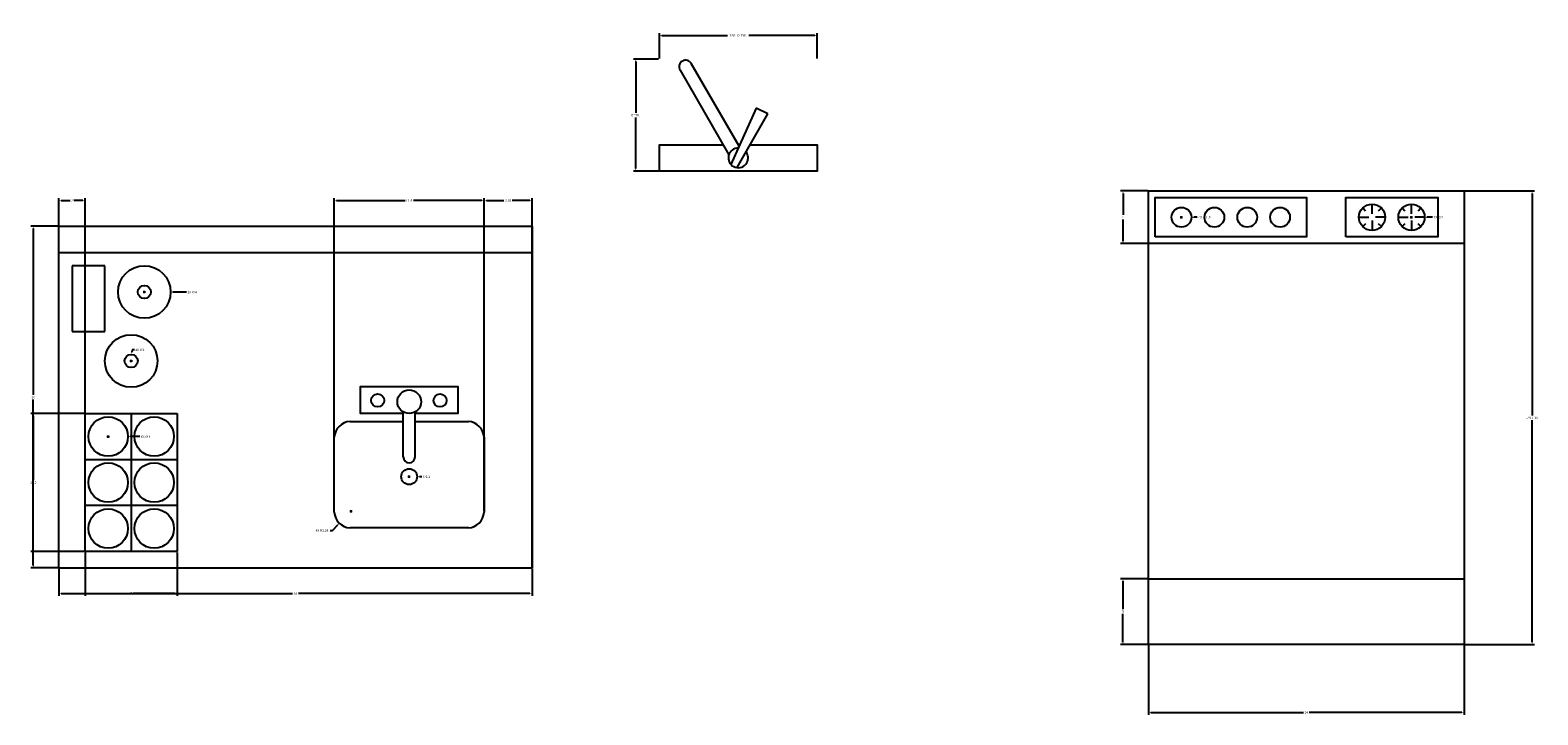
# Model space of a CAD drawing. Units: inches. Extents: x 821 to 2399, y 74 to 823.
# Tile 11 of 13: x 2026 to 2141, y 392 to 444. Entities that reach past the tile are written whole.
import ezdxf

# ---------------------------------------------------------------- set-up
doc = ezdxf.new("R2010")
doc.units = ezdxf.units.IN
doc.header["$MEASUREMENT"] = 0
doc.layers.get('0').update_dxf_attribs({"lineweight": 53})
for name, color, linetype, lineweight in [('A-ANNO-DIMS', 2, 'Continuous', 18), ('A-EQPM', 9, 'Continuous', 25), ('A-FLOR-CASE', 9, 'Continuous', 25), ('A-FLOR-FIXT', 8, 'Continuous', 25)]:
    doc.layers.add(name, color=color, linetype=linetype, lineweight=lineweight)
doc.styles.get("Standard").update_dxf_attribs({"font": 'arial.ttf'})
doc.dimstyles.get("Standard").update_dxf_attribs({"dimtxt": 0.18, "dimasz": 0.18, "dimexe": 0.18, "dimexo": 0.0625, "dimgap": 0.09, "dimtad": 0, "dimtih": 1, "dimtoh": 1, "dimdec": 4, "dimzin": 0, "dimdsep": 46, "dimtxsty": 'Standard', "dimcen": 0.09, "dimadec": 0, "dimazin": 0, "dimtfac": 1, "dimtdec": 4, "dimtofl": 0, "dimtmove": 0, "dimatfit": 3, "dimfxl": 1, "dimtolj": 1, "dimtzin": 0, "dimarcsym": 0})

# ---------------------------------------------------------------- blocks, each defined once
blk = doc.blocks.new('Faucet - single handle top')
for p, q in [((0.08, -0.26), (-2.26, -4.34)), ((-1.37, -4.79), (0.55, -0.5)), ((-0.06, -1.9), (3.57, -8.18)), ((4.43, -7.68), (0.72, -1.24)), ((-2.26, -4.34), (-1.37, -4.79))]:
    blk.add_line(p, q)
for points in [[(-0.92, -2), (-6, -2), (-6, 0), (6, 0), (6, -2), (1.16, -2)], [(-0.01, -2), (-0.12, -2)]]:
    blk.add_lwpolyline(points)
for centre, radius, start, end in [((0, -1), 0.75, 269.2246, 216.2304), ((4, -7.93), 0.5, 210, 30)]:
    blk.add_arc(centre, radius, start, end)
blk = doc.blocks.new('Dishwasher')
for p, q in [((17, 32.75), (17, 33.5)), ((20, 32.75), (20, 33.5)), ((16, 32.5), (16.75, 32.5)), ((16.3156, 33.1843), (16.5, 33)), ((17, 32.25), (17, 31.5)), ((18, 32.5), (17.25, 32.5)), ((17.5, 33), (17.6938, 33.1938)), ((19, 32.5), (19.75, 32.5)), ((19.3156, 33.1843), (19.5, 33)), ((20, 32.25), (20, 31.5)), ((21, 32.5), (20.25, 32.5)), ((20.5, 33), (20.6938, 33.1938)), ((16.5, 32), (16.2942, 31.7942)), ((17.7061, 31.7939), (17.5, 32)), ((19.5, 32), (19.2942, 31.7942)), ((20.7061, 31.7939), (20.5, 32)), ((24, 30.5), (0, 30.5)), ((0, 5), (24, 5))]:
    blk.add_line(p, q)
for points in [[(0, 0), (0, 34.5), (24, 34.5), (24, 0)], [(0.5, 31), (0.5, 34), (12, 34), (12, 31)], [(15, 31), (15, 34), (22, 34), (22, 31)]]:
    blk.add_lwpolyline(points, close=True)
for centre, radius in [((17, 32.5), 1), ((20, 32.5), 1), ((2.5, 32.5), 0.75), ((5, 32.5), 0.75), ((7.5, 32.5), 0.75), ((10, 32.5), 0.75)]:
    blk.add_circle(centre, radius)
blk = doc.blocks.new('*D36')
at = {"layer": 'A-ANNO-DIMS', "color": 0, "lineweight": -2, "transparency": 16777216}
for p, q in [((2074.05, 441.47), (2074.05, 443.39)), ((2074.23, 443.21), (2079.24, 443.21)), ((2085.87, 443.21), (2080.86, 443.21)), ((2086.05, 441.47), (2086.05, 443.39))]:
    blk.add_line(p, q, dxfattribs=at)
at = {"layer": 'A-ANNO-DIMS', "color": 0, "lineweight": 50, "transparency": 16777216}
for points in [[(2074.23, 443.24), (2074.23, 443.18), (2074.05, 443.21)], [(2085.87, 443.24), (2085.87, 443.18), (2086.05, 443.21)]]:
    blk.add_solid(points, dxfattribs=at)
at = {"layer": 'Defpoints', "color": 0, "lineweight": 50, "transparency": 16777216}
for p in [(2074.05, 443.21), (2074.05, 441.41), (2086.05, 441.41)]:
    blk.add_point(p, dxfattribs=at)
at = {"layer": 'A-ANNO-DIMS', "color": 0, "transparency": 16777216, "insert": (2080.05, 443.21), "char_height": 0.18, "attachment_point": 5}
blk.add_mtext('\\A1;TAP 12 TYP.', dxfattribs=at)
blk = doc.blocks.new('*D37')
at = {"layer": 'A-ANNO-DIMS', "color": 0, "lineweight": -2, "transparency": 16777216}
for p, q in [((2073.98, 441.41), (2072.07, 441.41)), ((2072.25, 441.23), (2072.25, 437.34)), ((2072.25, 433.09), (2072.25, 436.98)), ((2073.98, 432.91), (2072.07, 432.91))]:
    blk.add_line(p, q, dxfattribs=at)
at = {"layer": 'A-ANNO-DIMS', "color": 0, "lineweight": 50, "transparency": 16777216}
for points in [[(2072.22, 441.23), (2072.28, 441.23), (2072.25, 441.41)], [(2072.22, 433.09), (2072.28, 433.09), (2072.25, 432.91)]]:
    blk.add_solid(points, dxfattribs=at)
at = {"layer": 'Defpoints', "color": 0, "lineweight": 50, "transparency": 16777216}
for p in [(2074.05, 441.41), (2072.25, 432.91), (2074.05, 432.91)]:
    blk.add_point(p, dxfattribs=at)
at = {"layer": 'A-ANNO-DIMS', "color": 0, "transparency": 16777216, "insert": (2072.25, 437.16), "char_height": 0.18, "attachment_point": 5}
blk.add_mtext('\\A1;8 TYP.', dxfattribs=at)
blk = doc.blocks.new('*D76')
at = {"layer": 'A-ANNO-DIMS', "color": 0, "lineweight": -2, "transparency": 16777216}
for p, q in [((2135.34, 431.39), (2140.63, 431.39)), ((2140.45, 431.21), (2140.45, 414.32)), ((2140.45, 397.07), (2140.45, 413.96)), ((2135.34, 396.89), (2140.63, 396.89))]:
    blk.add_line(p, q, dxfattribs=at)
at = {"layer": 'A-ANNO-DIMS', "color": 0, "lineweight": 50, "transparency": 16777216}
for points in [[(2140.42, 431.21), (2140.48, 431.21), (2140.45, 431.39)], [(2140.42, 397.07), (2140.48, 397.07), (2140.45, 396.89)]]:
    blk.add_solid(points, dxfattribs=at)
at = {"layer": 'Defpoints', "color": 0, "lineweight": 50, "transparency": 16777216}
for p in [(2135.27, 431.39), (2140.45, 431.39), (2135.27, 396.89)]:
    blk.add_point(p, dxfattribs=at)
at = {"layer": 'A-ANNO-DIMS', "color": 0, "transparency": 16777216, "insert": (2140.45, 414.14), "char_height": 0.18, "attachment_point": 5}
blk.add_mtext('\\A1;UNIT 35', dxfattribs=at)
blk = doc.blocks.new('*D77')
at = {"layer": 'A-ANNO-DIMS', "color": 0, "lineweight": -2, "transparency": 16777216}
for p, q in [((2111.27, 396.83), (2111.27, 391.54)), ((2135.27, 396.83), (2135.27, 391.54)), ((2111.45, 391.72), (2123.05, 391.72)), ((2135.09, 391.72), (2123.49, 391.72))]:
    blk.add_line(p, q, dxfattribs=at)
at = {"layer": 'A-ANNO-DIMS', "color": 0, "lineweight": 50, "transparency": 16777216}
for points in [[(2111.45, 391.75), (2111.45, 391.69), (2111.27, 391.72)], [(2135.09, 391.75), (2135.09, 391.69), (2135.27, 391.72)]]:
    blk.add_solid(points, dxfattribs=at)
at = {"layer": 'Defpoints', "color": 0, "lineweight": 50, "transparency": 16777216}
for p in [(2111.27, 396.89), (2135.27, 396.89), (2135.27, 391.72)]:
    blk.add_point(p, dxfattribs=at)
at = {"layer": 'A-ANNO-DIMS', "color": 0, "transparency": 16777216, "insert": (2123.27, 391.72), "char_height": 0.18, "attachment_point": 5}
blk.add_mtext('\\A1;24', dxfattribs=at)
blk = doc.blocks.new('*D109')
at = {"layer": 'A-ANNO-DIMS', "color": 0, "lineweight": -2, "transparency": 16777216}
for p, q in [((2028.36, 402.64), (2028.36, 400.58)), ((2064.36, 402.64), (2064.36, 400.58)), ((2028.54, 400.76), (2046.14, 400.76)), ((2064.18, 400.76), (2046.58, 400.76))]:
    blk.add_line(p, q, dxfattribs=at)
at = {"layer": 'A-ANNO-DIMS', "color": 0, "lineweight": 50, "transparency": 16777216}
for points in [[(2028.54, 400.79), (2028.54, 400.73), (2028.36, 400.76)], [(2064.18, 400.79), (2064.18, 400.73), (2064.36, 400.76)]]:
    blk.add_solid(points, dxfattribs=at)
at = {"layer": 'Defpoints', "color": 0, "lineweight": 50, "transparency": 16777216}
for p in [(2028.36, 402.71), (2064.36, 402.71), (2064.36, 400.76)]:
    blk.add_point(p, dxfattribs=at)
at = {"layer": 'A-ANNO-DIMS', "color": 0, "transparency": 16777216, "insert": (2046.36, 400.76), "char_height": 0.18, "attachment_point": 5}
blk.add_mtext('\\A1;36', dxfattribs=at)
blk = doc.blocks.new('*D110')
at = {"layer": 'A-ANNO-DIMS', "color": 0, "lineweight": -2, "transparency": 16777216}
for p, q in [((2028.3, 428.71), (2026.23, 428.71)), ((2026.41, 428.53), (2026.41, 415.89)), ((2026.41, 402.89), (2026.41, 415.52)), ((2028.3, 402.71), (2026.23, 402.71))]:
    blk.add_line(p, q, dxfattribs=at)
at = {"layer": 'A-ANNO-DIMS', "color": 0, "lineweight": 50, "transparency": 16777216}
for points in [[(2026.38, 428.53), (2026.44, 428.53), (2026.41, 428.71)], [(2026.38, 402.89), (2026.44, 402.89), (2026.41, 402.71)]]:
    blk.add_solid(points, dxfattribs=at)
at = {"layer": 'Defpoints', "color": 0, "lineweight": 50, "transparency": 16777216}
for p in [(2026.41, 428.71), (2028.36, 428.71), (2028.36, 402.71)]:
    blk.add_point(p, dxfattribs=at)
at = {"layer": 'A-ANNO-DIMS', "color": 0, "transparency": 16777216, "insert": (2026.41, 415.71), "char_height": 0.18, "attachment_point": 5}
blk.add_mtext('\\A1;26', dxfattribs=at)
blk = doc.blocks.new('*D111')
at = {"layer": 'A-ANNO-DIMS', "color": 0, "lineweight": -2, "transparency": 16777216}
for p, q in [((2028.36, 402.77), (2028.36, 430.84)), ((2028.54, 430.66), (2029.21, 430.66)), ((2030.18, 430.66), (2029.51, 430.66)), ((2030.36, 404.02), (2030.36, 430.84))]:
    blk.add_line(p, q, dxfattribs=at)
at = {"layer": 'A-ANNO-DIMS', "color": 0, "lineweight": 50, "transparency": 16777216}
for points in [[(2028.54, 430.69), (2028.54, 430.63), (2028.36, 430.66)], [(2030.18, 430.69), (2030.18, 430.63), (2030.36, 430.66)]]:
    blk.add_solid(points, dxfattribs=at)
at = {"layer": 'Defpoints', "color": 0, "lineweight": 50, "transparency": 16777216}
for p in [(2030.36, 430.66), (2030.36, 403.96), (2028.36, 402.71)]:
    blk.add_point(p, dxfattribs=at)
at = {"layer": 'A-ANNO-DIMS', "color": 0, "transparency": 16777216, "insert": (2029.36, 430.66), "char_height": 0.18, "attachment_point": 5}
blk.add_mtext('\\A1;2', dxfattribs=at)
blk = doc.blocks.new('*D112')
at = {"layer": 'A-ANNO-DIMS', "color": 0, "lineweight": -2, "transparency": 16777216}
for p, q in [((2030.36, 403.89), (2030.36, 400.58)), ((2037.36, 403.89), (2037.36, 400.58)), ((2030.54, 400.76), (2033.72, 400.76)), ((2037.18, 400.76), (2034.01, 400.76))]:
    blk.add_line(p, q, dxfattribs=at)
at = {"layer": 'A-ANNO-DIMS', "color": 0, "lineweight": 50, "transparency": 16777216}
for points in [[(2030.54, 400.79), (2030.54, 400.73), (2030.36, 400.76)], [(2037.18, 400.79), (2037.18, 400.73), (2037.36, 400.76)]]:
    blk.add_solid(points, dxfattribs=at)
at = {"layer": 'Defpoints', "color": 0, "lineweight": 50, "transparency": 16777216}
for p in [(2030.36, 403.96), (2037.36, 403.96), (2037.36, 400.76)]:
    blk.add_point(p, dxfattribs=at)
at = {"layer": 'A-ANNO-DIMS', "color": 0, "transparency": 16777216, "insert": (2033.86, 400.76), "char_height": 0.18, "attachment_point": 5}
blk.add_mtext('\\A1;7', dxfattribs=at)
blk = doc.blocks.new('*D113')
at = {"layer": 'A-ANNO-DIMS', "color": 0, "lineweight": -2, "transparency": 16777216}
for p, q in [((2030.3, 414.46), (2026.23, 414.46)), ((2026.41, 414.28), (2026.41, 409.39)), ((2026.41, 404.14), (2026.41, 409.02)), ((2030.3, 403.96), (2026.23, 403.96))]:
    blk.add_line(p, q, dxfattribs=at)
at = {"layer": 'A-ANNO-DIMS', "color": 0, "lineweight": 50, "transparency": 16777216}
for points in [[(2026.38, 414.28), (2026.44, 414.28), (2026.41, 414.46)], [(2026.38, 404.14), (2026.44, 404.14), (2026.41, 403.96)]]:
    blk.add_solid(points, dxfattribs=at)
at = {"layer": 'Defpoints', "color": 0, "lineweight": 50, "transparency": 16777216}
for p in [(2026.41, 414.46), (2030.36, 414.46), (2030.36, 403.96)]:
    blk.add_point(p, dxfattribs=at)
at = {"layer": 'A-ANNO-DIMS', "color": 0, "transparency": 16777216, "insert": (2026.41, 409.21), "char_height": 0.18, "attachment_point": 5}
blk.add_mtext('\\A1;10.5', dxfattribs=at)
blk = doc.blocks.new('*D114')
at = {"layer": 'A-ANNO-DIMS', "color": 0, "lineweight": -2, "transparency": 16777216}
for p, q in [((2049.31, 407.02), (2049.31, 430.84)), ((2049.49, 430.66), (2054.7, 430.66)), ((2060.53, 430.66), (2055.33, 430.66)), ((2060.71, 407.02), (2060.71, 430.84))]:
    blk.add_line(p, q, dxfattribs=at)
at = {"layer": 'A-ANNO-DIMS', "color": 0, "lineweight": 50, "transparency": 16777216}
for points in [[(2049.49, 430.69), (2049.49, 430.63), (2049.31, 430.66)], [(2060.53, 430.69), (2060.53, 430.63), (2060.71, 430.66)]]:
    blk.add_solid(points, dxfattribs=at)
at = {"layer": 'Defpoints', "color": 0, "lineweight": 50, "transparency": 16777216}
for p in [(2060.71, 430.66), (2049.31, 406.96), (2060.71, 406.96)]:
    blk.add_point(p, dxfattribs=at)
at = {"layer": 'A-ANNO-DIMS', "color": 0, "transparency": 16777216, "insert": (2055.01, 430.66), "char_height": 0.18, "attachment_point": 5}
blk.add_mtext('\\A1;11.4', dxfattribs=at)
blk = doc.blocks.new('*D115')
at = {"layer": 'A-ANNO-DIMS', "color": 0, "lineweight": -2, "transparency": 16777216}
for p, q in [((2060.71, 407.02), (2060.71, 430.84)), ((2060.89, 430.66), (2062.21, 430.66)), ((2064.18, 430.66), (2062.86, 430.66)), ((2064.36, 402.77), (2064.36, 430.84))]:
    blk.add_line(p, q, dxfattribs=at)
at = {"layer": 'A-ANNO-DIMS', "color": 0, "lineweight": 50, "transparency": 16777216}
for points in [[(2060.89, 430.69), (2060.89, 430.63), (2060.71, 430.66)], [(2064.18, 430.69), (2064.18, 430.63), (2064.36, 430.66)]]:
    blk.add_solid(points, dxfattribs=at)
at = {"layer": 'Defpoints', "color": 0, "lineweight": 50, "transparency": 16777216}
for p in [(2064.36, 430.66), (2060.71, 406.96), (2064.36, 402.71)]:
    blk.add_point(p, dxfattribs=at)
at = {"layer": 'A-ANNO-DIMS', "color": 0, "transparency": 16777216, "insert": (2062.54, 430.66), "char_height": 0.18, "attachment_point": 5}
blk.add_mtext('\\A1;3.65', dxfattribs=at)
blk = doc.blocks.new('*D116')
at = {"layer": 'A-ANNO-DIMS', "color": 0, "lineweight": -2, "transparency": 16777216}
for p, q in [((2111.210277, 431.390534), (2109.142777, 431.390534)), ((2109.322777, 431.210534), (2109.322777, 429.570534)), ((2109.322777, 427.570534), (2109.322777, 429.210534)), ((2111.210277, 427.390534), (2109.142777, 427.390534))]:
    blk.add_line(p, q, dxfattribs=at)
at = {"layer": 'A-ANNO-DIMS', "color": 0, "lineweight": 50, "transparency": 16777216}
for points in [[(2109.292777, 431.210534), (2109.352777, 431.210534), (2109.322777, 431.390534)], [(2109.292777, 427.570534), (2109.352777, 427.570534), (2109.322777, 427.390534)]]:
    blk.add_solid(points, dxfattribs=at)
at = {"layer": 'Defpoints', "color": 0, "lineweight": 50, "transparency": 16777216}
for p in [(2109.322777, 431.390534), (2111.272777, 431.390534), (2111.272777, 427.390534)]:
    blk.add_point(p, dxfattribs=at)
at = {"layer": 'A-ANNO-DIMS', "color": 0, "transparency": 16777216, "insert": (2109.322777, 429.390534), "char_height": 0.18, "attachment_point": 5}
blk.add_mtext('\\A1;4', dxfattribs=at)
blk = doc.blocks.new('*D117')
at = {"layer": 'A-ANNO-DIMS', "color": 0, "lineweight": -2, "transparency": 16777216}
for p, q in [((2111.21, 401.89), (2109.14, 401.89)), ((2109.32, 401.71), (2109.32, 399.57)), ((2109.32, 397.07), (2109.32, 399.21)), ((2111.21, 396.89), (2109.14, 396.89))]:
    blk.add_line(p, q, dxfattribs=at)
at = {"layer": 'A-ANNO-DIMS', "color": 0, "lineweight": 50, "transparency": 16777216}
for points in [[(2109.29, 401.71), (2109.35, 401.71), (2109.32, 401.89)], [(2109.29, 397.07), (2109.35, 397.07), (2109.32, 396.89)]]:
    blk.add_solid(points, dxfattribs=at)
at = {"layer": 'Defpoints', "color": 0, "lineweight": 50, "transparency": 16777216}
for p in [(2109.32, 401.89), (2111.27, 401.89), (2111.27, 396.89)]:
    blk.add_point(p, dxfattribs=at)
at = {"layer": 'A-ANNO-DIMS', "color": 0, "transparency": 16777216, "insert": (2109.32, 399.39), "char_height": 0.18, "attachment_point": 5}
blk.add_mtext('\\A1;5', dxfattribs=at)
blk = doc.blocks.new('*D143')
at = {"layer": 'A-ANNO-DIMS', "color": 0, "lineweight": -2, "transparency": 16777216}
for p, q in [((2034.77, 423.71), (2034.95, 423.71)), ((2034.86, 423.62), (2034.86, 423.8)), ((2038.06, 423.7), (2037.04, 423.7))]:
    blk.add_line(p, q, dxfattribs=at)
at = {"layer": 'A-ANNO-DIMS', "color": 0, "lineweight": 50, "transparency": 16777216}
blk.add_solid([(2037.04, 423.73), (2037.04, 423.67), (2036.86, 423.7)], dxfattribs=at)
at = {"layer": 'Defpoints', "color": 0, "lineweight": 50, "transparency": 16777216}
for p in [(2032.86, 423.71), (2036.86, 423.7)]:
    blk.add_point(p, dxfattribs=at)
at = {"layer": 'A-ANNO-DIMS', "color": 0, "transparency": 16777216, "insert": (2038.5, 423.7), "char_height": 0.18, "attachment_point": 5}
blk.add_mtext('\\A1;2X ∅4', dxfattribs=at)
blk = doc.blocks.new('*D144')
at = {"layer": 'A-ANNO-DIMS', "color": 0, "lineweight": -2, "transparency": 16777216}
for p, q in [((2033.93, 419.31), (2033.91, 419.13)), ((2034.11, 419.31), (2033.93, 419.31)), ((2033.77, 418.46), (2033.95, 418.46)), ((2033.86, 418.37), (2033.86, 418.55))]:
    blk.add_line(p, q, dxfattribs=at)
at = {"layer": 'A-ANNO-DIMS', "color": 0, "lineweight": 50, "transparency": 16777216}
blk.add_solid([(2033.88, 419.14), (2033.94, 419.13), (2033.9, 418.96)], dxfattribs=at)
at = {"layer": 'Defpoints', "color": 0, "lineweight": 50, "transparency": 16777216}
for p in [(2033.9, 418.96), (2033.83, 417.96)]:
    blk.add_point(p, dxfattribs=at)
at = {"layer": 'A-ANNO-DIMS', "color": 0, "transparency": 16777216, "insert": (2034.53, 419.31), "char_height": 0.18, "attachment_point": 5}
blk.add_mtext('\\A1;4X ∅1', dxfattribs=at)
blk = doc.blocks.new('*D145')
at = {"layer": 'A-ANNO-DIMS', "color": 0, "lineweight": -2, "transparency": 16777216}
for p, q in [((2032.02, 412.71), (2032.2, 412.71)), ((2032.11, 412.62), (2032.11, 412.8)), ((2034.51, 412.7), (2033.79, 412.7))]:
    blk.add_line(p, q, dxfattribs=at)
at = {"layer": 'A-ANNO-DIMS', "color": 0, "lineweight": 50, "transparency": 16777216}
blk.add_solid([(2033.79, 412.73), (2033.79, 412.67), (2033.61, 412.7)], dxfattribs=at)
at = {"layer": 'Defpoints', "color": 0, "lineweight": 50, "transparency": 16777216}
for p in [(2030.61, 412.71), (2033.61, 412.7)]:
    blk.add_point(p, dxfattribs=at)
at = {"layer": 'A-ANNO-DIMS', "color": 0, "transparency": 16777216, "insert": (2034.95, 412.7), "char_height": 0.18, "attachment_point": 5}
blk.add_mtext('\\A1;6X ∅3', dxfattribs=at)
blk = doc.blocks.new('*D146')
at = {"layer": 'A-ANNO-DIMS', "color": 0, "lineweight": -2, "transparency": 16777216}
for p, q in [((2054.92, 409.66), (2055.1, 409.66)), ((2055.01, 409.57), (2055.01, 409.75)), ((2055.97, 409.65), (2055.79, 409.65))]:
    blk.add_line(p, q, dxfattribs=at)
at = {"layer": 'A-ANNO-DIMS', "color": 0, "lineweight": 50, "transparency": 16777216}
blk.add_solid([(2055.79, 409.68), (2055.79, 409.62), (2055.61, 409.65)], dxfattribs=at)
at = {"layer": 'Defpoints', "color": 0, "lineweight": 50, "transparency": 16777216}
for p in [(2054.41, 409.66), (2055.61, 409.65)]:
    blk.add_point(p, dxfattribs=at)
at = {"layer": 'A-ANNO-DIMS', "color": 0, "transparency": 16777216, "insert": (2056.32, 409.65), "char_height": 0.18, "attachment_point": 5}
blk.add_mtext('\\A1;∅1.2', dxfattribs=at)
blk = doc.blocks.new('*D147')
at = {"layer": 'A-ANNO-DIMS', "color": 0, "lineweight": -2, "transparency": 16777216}
for p, q in [((2050.5, 407.03), (2050.68, 407.03)), ((2050.59, 406.94), (2050.59, 407.12)), ((2048.99, 405.56), (2049.17, 405.56)), ((2049.17, 405.56), (2049.58, 405.98))]:
    blk.add_line(p, q, dxfattribs=at)
at = {"layer": 'A-ANNO-DIMS', "color": 0, "lineweight": 50, "transparency": 16777216}
blk.add_solid([(2049.55, 406), (2049.6, 405.96), (2049.7, 406.11)], dxfattribs=at)
at = {"layer": 'Defpoints', "color": 0, "lineweight": 50, "transparency": 16777216}
for p in [(2049.7, 406.11), (2050.59, 407.03)]:
    blk.add_point(p, dxfattribs=at)
at = {"layer": 'A-ANNO-DIMS', "color": 0, "transparency": 16777216, "insert": (2048.38, 405.56), "char_height": 0.18, "attachment_point": 5}
blk.add_mtext('\\A1;4X R1.28', dxfattribs=at)
blk = doc.blocks.new('*D148')
at = {"layer": 'A-ANNO-DIMS', "color": 0, "lineweight": -2, "transparency": 16777216}
for p, q in [((2113.68, 429.39), (2113.86, 429.39)), ((2113.77, 429.3), (2113.77, 429.48)), ((2114.97, 429.39), (2114.7, 429.39))]:
    blk.add_line(p, q, dxfattribs=at)
at = {"layer": 'A-ANNO-DIMS', "color": 0, "lineweight": 50, "transparency": 16777216}
blk.add_solid([(2114.7, 429.42), (2114.7, 429.36), (2114.52, 429.39)], dxfattribs=at)
at = {"layer": 'Defpoints', "color": 0, "lineweight": 50, "transparency": 16777216}
for p in [(2113.02, 429.39), (2114.52, 429.39)]:
    blk.add_point(p, dxfattribs=at)
at = {"layer": 'A-ANNO-DIMS', "color": 0, "transparency": 16777216, "insert": (2115.52, 429.39), "char_height": 0.18, "attachment_point": 5}
blk.add_mtext('\\A1;4X ∅1.5', dxfattribs=at)
blk = doc.blocks.new('*D149')
at = {"layer": 'A-ANNO-DIMS', "color": 0, "lineweight": -2, "transparency": 16777216}
for p, q in [((2131.18, 429.39), (2131.36, 429.39)), ((2131.27, 429.3), (2131.27, 429.48)), ((2132.87, 429.39), (2132.45, 429.39))]:
    blk.add_line(p, q, dxfattribs=at)
at = {"layer": 'A-ANNO-DIMS', "color": 0, "lineweight": 50, "transparency": 16777216}
blk.add_solid([(2132.45, 429.42), (2132.45, 429.36), (2132.27, 429.39)], dxfattribs=at)
at = {"layer": 'Defpoints', "color": 0, "lineweight": 50, "transparency": 16777216}
for p in [(2130.27, 429.39), (2132.27, 429.39)]:
    blk.add_point(p, dxfattribs=at)
at = {"layer": 'A-ANNO-DIMS', "color": 0, "transparency": 16777216, "insert": (2133.31, 429.39), "char_height": 0.18, "attachment_point": 5}
blk.add_mtext('\\A1;2X ∅2', dxfattribs=at)

msp = doc.modelspace()

# ---------------------------------------------------------------- linework, layer by layer
at = {"layer": 'A-FLOR-CASE'}
for p, q in [((2028.3633, 428.7065), (2064.3633, 428.7065)), ((2028.3633, 402.7065), (2028.3633, 428.7065)), ((2064.3633, 428.7065), (2064.3633, 402.7065)), ((2028.3633, 426.7065), (2064.3633, 426.7065)), ((2031.8633, 425.7065), (2029.3633, 425.7065)), ((2029.3633, 425.7065), (2029.3633, 420.7065)), ((2031.8633, 420.7065), (2031.8633, 425.7065)), ((2029.3633, 420.7065), (2031.8633, 420.7065)), ((2030.3633, 414.4565), (2037.3633, 414.4565)), ((2030.3633, 403.9565), (2030.3633, 414.4565)), ((2033.8633, 414.4565), (2033.8633, 403.9565)), ((2037.3633, 414.4565), (2037.3633, 403.9565)), ((2030.3633, 410.9565), (2037.3633, 410.9565)), ((2037.3633, 407.4565), (2030.3633, 407.4565)), ((2037.3633, 403.9565), (2030.3633, 403.9565)), ((2064.3633, 402.7065), (2028.3633, 402.7065))]:
    msp.add_line(p, q, dxfattribs=at)
for centre, radius in [((2034.8633, 423.7065), 2), ((2034.8633, 423.7065), 0.5), ((2033.8633, 418.4565), 2), ((2033.8633, 418.4565), 0.5), ((2032.1133, 412.7065), 1.5), ((2035.6133, 412.7065), 1.5), ((2032.1133, 409.2065), 1.5), ((2035.6133, 409.2065), 1.5), ((2032.1133, 405.7065), 1.5), ((2035.6133, 405.7065), 1.5)]:
    msp.add_circle(centre, radius, dxfattribs=at)
at = {"layer": 'A-FLOR-FIXT'}
for p, q in [((2054.5633, 411.1565), (2054.5633, 414.5781)), ((2055.4634, 411.1565), (2055.4634, 414.5781))]:
    msp.add_line(p, q, dxfattribs=at)
for points in [[(2054.5633, 414.4565), (2051.3133, 414.4565), (2051.3133, 416.5065), (2055.1133, 416.5065)], [(2055.112, 416.5065), (2058.7134, 416.5065), (2058.7134, 414.4565), (2055.4634, 414.4565)], [(2050.5133, 413.8565), (2054.5633, 413.8565)], [(2055.4634, 413.8565), (2059.5133, 413.8565)], [(2049.3133, 406.9565), (2049.3133, 412.6565)], [(2060.7134, 412.6565), (2060.7134, 406.9565)], [(2059.5133, 405.7565), (2050.5133, 405.7565)]]:
    msp.add_lwpolyline(points, dxfattribs=at)
for centre, radius in [((2052.6133, 415.4565), 0.5), ((2055.0133, 415.3565), 0.9), ((2057.3633, 415.4565), 0.5), ((2055.0133, 409.6565), 0.6)]:
    msp.add_circle(centre, radius, dxfattribs=at)
for centre, radius, start, end in [((2050.5884, 412.5815), 1.2772, 93.36646, 176.6335), ((2059.4383, 412.5815), 1.2772, 3.366461, 86.63354), ((2055.0133, 411.1565), 0.45, 180, 0), ((2050.5884, 407.0315), 1.2772, 183.3665, 266.6335), ((2059.4383, 407.0315), 1.2772, 273.3665, 356.6335)]:
    msp.add_arc(centre, radius, start, end, dxfattribs=at)

# ---------------------------------------------------------------- block references
at = {"layer": 'A-EQPM'}
msp.add_blockref('Dishwasher', (2111.2728, 396.8905), dxfattribs=at)
at = {"layer": 'A-FLOR-FIXT', "rotation": 180}
msp.add_blockref('Faucet - single handle top', (2080.0474, 432.9086), dxfattribs=at)

# ---------------------------------------------------------------- dimensions: what is measured, and where the dimension line sits
at = {"layer": 'A-ANNO-DIMS'}
for base, p1, p2, angle, text, picture, middle in [((2074.0474, 443.2079), (2086.0474, 441.4079), (2074.0474, 441.4079), 180, 'TAP <> TYP.', '*D36', (2080.0474, 443.2079)), ((2072.2474, 432.9086), (2074.0474, 441.4079), (2074.0474, 432.9086), 270, '<> TYP.', '*D37', (2072.2474, 437.1582)), ((2140.447776791, 431.3905341671), (2135.272776791, 396.8905341671), (2135.272776791, 431.3905341671), 90, 'UNIT <>', '*D76', (2140.447776791, 414.1405341671))]:
    dim = msp.add_linear_dim(base=base, p1=p1, p2=p2, angle=angle, text=text, dimstyle='Standard', override={"dimdec": 0, "dimlfac": 1, "dimrnd": 0, "dimzin": 0, "dimdsep": 46, "dimlunit": 2}, dxfattribs=at)
    dim.commit()
    dim.dimension.update_dxf_attribs({"geometry": picture, "text_midpoint": middle})
for base, p1, p2, override, picture, middle in [((2109.3228, 431.3905), (2111.2728, 427.3905), (2111.2728, 431.3905), {"dimdec": 0, "dimlfac": 1, "dimrnd": 0, "dimzin": 0, "dimdsep": 46, "dimlunit": 2}, '*D116', (2109.3228, 429.3905)), ((2026.4133, 428.7065), (2028.3633, 402.7065), (2028.3633, 428.7065), {"dimdec": 0, "dimlfac": 1, "dimrnd": 0, "dimzin": 0, "dimdsep": 46, "dimlunit": 2}, '*D110', (2026.4133, 415.7065)), ((2026.4133, 414.4565), (2030.3633, 403.9565), (2030.3633, 414.4565), {"dimdec": 1, "dimlfac": 1, "dimrnd": 0, "dimzin": 0, "dimdsep": 46, "dimlunit": 2}, '*D113', (2026.4133, 409.2065)), ((2109.3228, 401.8905), (2111.2728, 396.8905), (2111.2728, 401.8905), {"dimdec": 0, "dimlfac": 1, "dimrnd": 0, "dimzin": 0, "dimdsep": 46, "dimlunit": 2}, '*D117', (2109.3228, 399.3905))]:
    dim = msp.add_linear_dim(base=base, p1=p1, p2=p2, angle=90, dimstyle='Standard', override=override, dxfattribs=at)
    dim.commit()
    dim.dimension.update_dxf_attribs({"geometry": picture, "text_midpoint": middle})
for base, p1, p2, override, picture, middle in [((2030.3633, 430.6565), (2028.3633, 402.7065), (2030.3633, 403.9565), {"dimdec": 0, "dimlfac": 1, "dimrnd": 0, "dimzin": 0, "dimdsep": 46, "dimlunit": 2}, '*D111', (2029.3633, 430.6565)), ((2060.7133, 430.6565), (2049.3133, 406.9565), (2060.7133, 406.9565), {"dimdec": 1, "dimlfac": 1, "dimrnd": 0, "dimzin": 0, "dimdsep": 46, "dimlunit": 2}, '*D114', (2055.0133, 430.6565)), ((2064.3633, 430.6565), (2060.7133, 406.9565), (2064.3633, 402.7065), {"dimdec": 2, "dimlfac": 1, "dimrnd": 0, "dimzin": 0, "dimdsep": 46, "dimlunit": 2}, '*D115', (2062.5383, 430.6565)), ((2037.3633, 400.7565), (2030.3633, 403.9565), (2037.3633, 403.9565), {"dimdec": 0, "dimlfac": 1, "dimrnd": 0, "dimzin": 0, "dimdsep": 46, "dimlunit": 2}, '*D112', (2033.8633, 400.7565)), ((2064.3633, 400.7565), (2028.3633, 402.7065), (2064.3633, 402.7065), {"dimdec": 0, "dimlfac": 1, "dimrnd": 0, "dimzin": 0, "dimdsep": 46, "dimlunit": 2}, '*D109', (2046.3633, 400.7565)), ((2135.2728, 391.7155), (2111.2728, 396.8905), (2135.2728, 396.8905), {"dimdec": 0, "dimlfac": 1, "dimrnd": 0, "dimzin": 0, "dimdsep": 46, "dimlunit": 2}, '*D77', (2123.2728, 391.7155))]:
    dim = msp.add_linear_dim(base=base, p1=p1, p2=p2, dimstyle='Standard', override=override, dxfattribs=at)
    dim.commit()
    dim.dimension.update_dxf_attribs({"geometry": picture, "text_midpoint": middle})
for p1, p2, text, override, picture, middle in [((2113.0228, 429.3911), (2114.5228, 429.39), '4X <>', {"dimdec": 1, "dimlfac": 1, "dimrnd": 0, "dimzin": 0, "dimdsep": 46, "dimlunit": 2}, '*D148', (2114.9728, 429.3897)), ((2130.2728, 429.3911), (2132.2728, 429.39), '2X <>', {"dimdec": 0, "dimlfac": 1, "dimrnd": 0, "dimzin": 0, "dimdsep": 46, "dimlunit": 2}, '*D149', (2132.8728, 429.3897)), ((2032.8634, 423.7132), (2036.8633, 423.6998), '2X <>', {"dimdec": 0, "dimlfac": 1, "dimrnd": 0, "dimzin": 0, "dimdsep": 46, "dimlunit": 2}, '*D143', (2038.0633, 423.6958)), ((2033.8263, 417.9579), (2033.9004, 418.9551), '4X <>', {"dimdec": 0, "dimlfac": 1, "dimrnd": 0, "dimzin": 0, "dimdsep": 46, "dimlunit": 2}, '*D144', (2034.5288, 419.3141)), ((2030.6134, 412.713), (2033.6133, 412.6999), '6X <>', {"dimdec": 0, "dimlfac": 1, "dimrnd": 0, "dimzin": 0, "dimdsep": 46, "dimlunit": 2}, '*D145', (2034.5133, 412.696))]:
    dim = msp.add_diameter_dim_2p(p1=p1, p2=p2, text=text, dimstyle='Standard', override=override, dxfattribs=at)
    dim.commit()
    dim.dimension.update_dxf_attribs({"geometry": picture, "text_midpoint": middle, "dimtype": 163})
dim = msp.add_diameter_dim_2p(p1=(2054.4134, 409.6631), p2=(2055.6133, 409.6499), dimstyle='Standard', override={"dimdec": 1, "dimlfac": 1, "dimrnd": 0, "dimzin": 0, "dimdsep": 46, "dimlunit": 2}, dxfattribs=at)
dim.commit()
dim.dimension.update_dxf_attribs({"geometry": '*D146', "text_midpoint": (2055.9733, 409.6459), "dimtype": 163})
dim = msp.add_radius_dim(center=(2050.5884, 407.0315), mpoint=(2049.7013, 406.1127), text='4X <>', dimstyle='Standard', override={"dimdec": 2, "dimlfac": 1, "dimrnd": 0, "dimzin": 0, "dimdsep": 46, "dimlunit": 2}, dxfattribs=at)
dim.commit()
dim.dimension.update_dxf_attribs({"geometry": '*D147', "text_midpoint": (2048.3818, 405.5615), "dimtype": 164})

doc.saveas('drawing.dxf')
